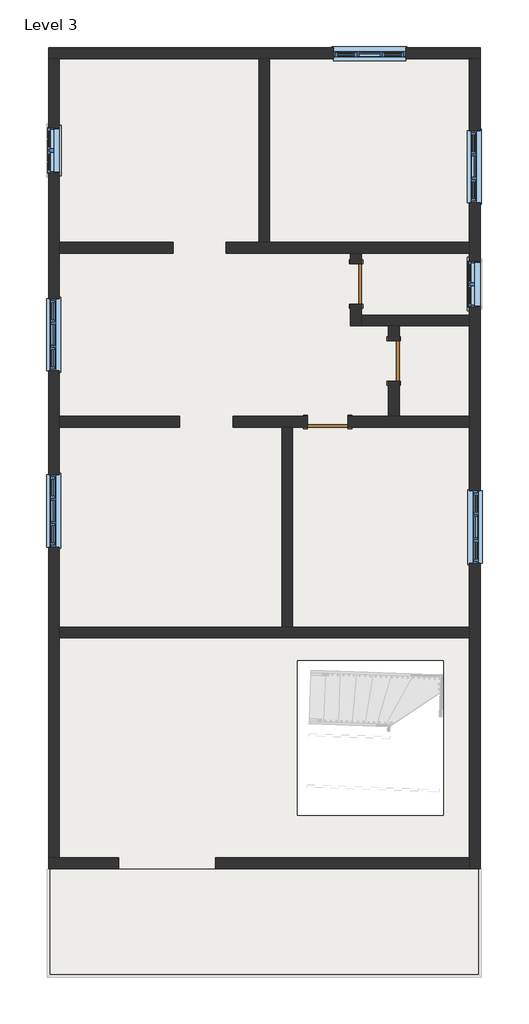
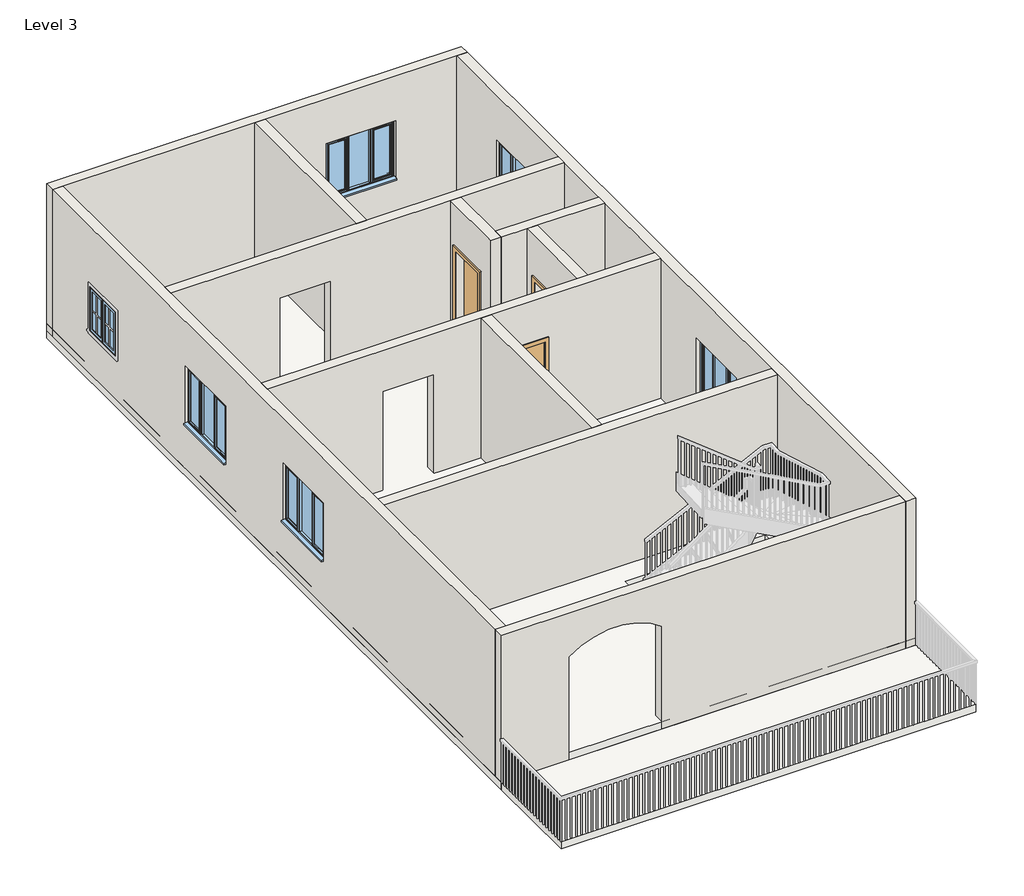
# One storey, part 1 of 3: 12 walls, 7 windows, 3 doors, 2 slabs, 1 roof.
"""IFC4 building model written with IfcOpenShell, lengths in millimetres."""

from ifc_helpers import new_model, si_unit, frame, origin, place, context, project, spatial, polyline, circle_curve, outline, extrude, faceted_brep, transform, mapped, element, save
from ifc_brep_helpers import plane_surface, revolved_surface, advanced_brep
from components import door_b6acaa4e, window_c29befe5, windows_tpl_plain_1360x1210mm_e2a6c9d8

model = new_model("IFC4")

# Units and contexts
model_context = context("Model", 3, world=origin())
ifc_project = project(units=[si_unit("LENGTHUNIT", "METRE", prefix="MILLI")], contexts=[model_context])

# Site, building, storey
site = spatial("IfcSite", under=ifc_project)
building = spatial("IfcBuilding", under=site)
storey = spatial("IfcBuildingStorey", under=building, Name="Level 3", Elevation=6096.0)

# Doors
placement = place(None, origin())
door_shape = door_b6acaa4e(model_context)
element("IfcDoor", 1, ObjectType="Single-Flush : 30\" x 84\"", at=placement, inside=storey, context=model_context, shape_type="MappedRepresentation", body=[
    mapped(door_shape, transform((-9158.3126504, 6947.728857, 6096.0), x_axis=(0.0, -1.0, 0.0), y_axis=(1.0, 0.0, 0.0), z_axis=(0.0, 0.0, 1.0))),
])
element("IfcDoor", 2, ObjectType="Single-Flush : 30\" x 84\"", at=placement, inside=storey, context=model_context, shape_type="MappedRepresentation", body=[
    mapped(door_shape, transform((-9691.7126504, 4356.928857, 6096.0), x_axis=(-1.0, 0.0, 0.0), y_axis=(0.0, -1.0, 0.0), z_axis=(0.0, 0.0, 1.0))),
])
element("IfcDoor", 3, ObjectType="Single-Flush : 30\" x 84\"", at=placement, inside=storey, context=model_context, shape_type="MappedRepresentation", body=[
    mapped(door_shape, transform((-8447.1126504, 5499.928857, 6096.0), x_axis=(0.0, -1.0, 0.0), y_axis=(1.0, 0.0, 0.0), z_axis=(0.0, 0.0, 1.0))),
])

# Roof
element("IfcRoof", 4, ObjectType="Generic - 12\"", at=placement, inside=storey, context=model_context, shape_type="SweptSolid", body=[
    extrude(outline(polyline([(-6821.5126504, -4050.471143), (-14949.5126504, -4050.471143), (-14949.5126504, 11392.728857), (-6821.5126504, 11392.728857), (-6821.5126504, -4050.471143)]), holes=[polyline([(-7518.4, -135.4836), (-10261.6, -135.4836), (-10261.6, -3048.381), (-7518.4, -3048.381), (-7518.4, -135.4836)])]), frame((0.0, 0.0, 6096.0), z_axis=(0.0, 0.0, 1.0), x_axis=(1.0, 0.0, 0.0)), (0.0, 0.0, 1.0), 152.4),
])

# Slabs
element("IfcSlab", 5, ObjectType="Generic - 12\"", at=placement, inside=storey, context=model_context, shape_type="SweptSolid", body=[
    extrude(outline(polyline([(-6821.5126504, 11392.728857), (-6821.5126504, -4050.471143), (-14949.5126504, -4050.471143), (-14949.5126504, 11392.728857), (-6821.5126504, 11392.728857)]), holes=[polyline([(-7518.4, -135.4836), (-10261.6, -135.4836), (-10261.6, -3048.381), (-7518.4, -3048.381), (-7518.4, -135.4836)])]), frame((0.0, 0.0, 5943.6), z_axis=(0.0, 0.0, 1.0), x_axis=(1.0, 0.0, 0.0)), (0.0, 0.0, 1.0), 152.4),
])
element("IfcSlab", 6, ObjectType="Generic - 12\"", at=placement, inside=storey, context=model_context, shape_type="SweptSolid", body=[
    extrude(outline(polyline([(-6821.5126504, -4050.471143), (-6821.5126504, -6082.471143), (-14949.5126504, -6082.471143), (-14949.5126504, -4050.471143), (-6821.5126504, -4050.471143)])), frame((0.0, 0.0, 5943.6), z_axis=(0.0, 0.0, 1.0), x_axis=(1.0, 0.0, 0.0)), (0.0, 0.0, 1.0), 152.4),
])

# Walls
element("IfcWall", 7, ObjectType="Generic - 4.5\" p", at=placement, inside=storey, context=model_context, shape_type="SweptSolid", body=[
    extrude(outline(polyline([(-10987.1126504, 7735.128857), (-10987.1126504, 11189.528857), (-10783.9126504, 11189.528857), (-10783.9126504, 7735.128857), (-10987.1126504, 7735.128857)])), frame((0.0, 0.0, 6096.0), z_axis=(0.0, 0.0, 1.0), x_axis=(1.0, 0.0, 0.0)), (0.0, 0.0, 1.0), 3048.0),
])
element("IfcWall", 8, ObjectType="Generic - 4.5\" p", at=placement, inside=storey, context=model_context, shape_type="Brep", body=[
    faceted_brep([(-7024.7126504, 7735.128857, 6096.0), (-10783.9126504, 7735.128857, 6096.0), (-10987.1126504, 7735.128857, 6096.0), (-11604.7126504, 7735.128857, 6096.0), (-11604.7126504, 7735.128857, 8296.0), (-12604.7126504, 7735.128857, 8296.0), (-12604.7126504, 7735.128857, 6096.0), (-14746.3126504, 7735.128857, 6096.0), (-14746.3126504, 7735.128857, 9144.0), (-10987.1126504, 7735.128857, 9144.0), (-10783.9126504, 7735.128857, 9144.0), (-7024.7126504, 7735.128857, 9144.0), (-11604.7126504, 7531.928857, 8296.0), (-11604.7126504, 7531.928857, 6096.0), (-9259.9126504, 7531.928857, 6096.0), (-9056.7126504, 7531.928857, 6096.0), (-7024.7126504, 7531.928857, 6096.0), (-7024.7126504, 7531.928857, 9144.0), (-9056.7126504, 7531.928857, 9144.0), (-9259.9126504, 7531.928857, 9144.0), (-14746.3126504, 7531.928857, 9144.0), (-14746.3126504, 7531.928857, 6096.0), (-12604.7126504, 7531.928857, 6096.0), (-12604.7126504, 7531.928857, 8296.0)], [[[0, 1, 2, 3, 4, 5, 6, 7, 8, 9, 10, 11]], [[12, 13, 14, 15, 16, 17, 18, 19, 20, 21, 22, 23]], [[22, 21, 7, 6]], [[16, 15, 14, 13, 3, 2, 1, 0]], [[11, 10, 9, 8, 20, 19, 18, 17]], [[8, 7, 21, 20]], [[0, 11, 17, 16]], [[4, 3, 13, 12]], [[5, 4, 12, 23]], [[6, 5, 23, 22]]]),
])
element("IfcWall", 9, ObjectType="Generic - 4.5\" p", at=placement, inside=storey, context=model_context, shape_type="Brep", body=[
    faceted_brep([(-9259.9126504, 6566.728857, 8229.6), (-9259.9126504, 6566.728857, 6096.0), (-9259.9126504, 6160.328857, 6096.0), (-9259.9126504, 6160.328857, 9144.0), (-9259.9126504, 7531.928857, 9144.0), (-9259.9126504, 7531.928857, 6096.0), (-9259.9126504, 7328.728857, 6096.0), (-9259.9126504, 7328.728857, 8229.6), (-9056.7126504, 6160.328857, 6096.0), (-9056.7126504, 6363.528857, 6096.0), (-9056.7126504, 6566.728857, 6096.0), (-9056.7126504, 6566.728857, 8229.6), (-9056.7126504, 7328.728857, 8229.6), (-9056.7126504, 7328.728857, 6096.0), (-9056.7126504, 7531.928857, 6096.0), (-9056.7126504, 7531.928857, 9144.0), (-9056.7126504, 6363.528857, 9144.0), (-9056.7126504, 6160.328857, 9144.0)], [[[0, 1, 2, 3, 4, 5, 6, 7]], [[8, 9, 10, 11, 12, 13, 14, 15, 16, 17]], [[6, 5, 14, 13]], [[2, 1, 10, 9, 8]], [[4, 3, 17, 16, 15]], [[5, 4, 15, 14]], [[3, 2, 8, 17]], [[11, 10, 1, 0]], [[12, 11, 0, 7]], [[13, 12, 7, 6]]]),
])
element("IfcWall", 10, ObjectType="Generic - 4.5\" p", at=placement, inside=storey, context=model_context, shape_type="Brep", body=[
    faceted_brep([(-9056.7126504, 6160.328857, 6096.0), (-8548.7126504, 6160.328857, 6096.0), (-8345.5126504, 6160.328857, 6096.0), (-7024.7126504, 6160.328857, 6096.0), (-7024.7126504, 6160.328857, 9144.0), (-8345.5126504, 6160.328857, 9144.0), (-8548.7126504, 6160.328857, 9144.0), (-9056.7126504, 6160.328857, 9144.0), (-9056.7126504, 6363.528857, 6096.0), (-9056.7126504, 6363.528857, 9144.0), (-7024.7126504, 6363.528857, 9144.0), (-7024.7126504, 6363.528857, 6096.0)], [[[0, 1, 2, 3, 4, 5, 6, 7]], [[8, 9, 10, 11]], [[3, 2, 1, 0, 8, 11]], [[7, 6, 5, 4, 10, 9]], [[0, 7, 9, 8]], [[4, 3, 11, 10]]]),
])
element("IfcWall", 11, ObjectType="Generic - 4.5\" p", at=placement, inside=storey, context=model_context, shape_type="SweptSolid", body=[
    extrude(outline(polyline([(5118.928857, 8229.6), (5118.928857, 6096.0), (4458.528857, 6096.0), (4458.528857, 9144.0), (6160.328857, 9144.0), (6160.328857, 6096.0), (5880.928857, 6096.0), (5880.928857, 8229.6), (5118.928857, 8229.6)])), frame((-8548.7126504, 0.0, 0.0), z_axis=(1.0, 0.0, 0.0), x_axis=(0.0, 1.0, 0.0)), (0.0, 0.0, 1.0), 203.2),
])
element("IfcWall", 12, ObjectType="Generic - 4.5\" p", at=placement, inside=storey, context=model_context, shape_type="Brep", body=[
    faceted_brep([(-10072.7126504, 4458.528857, 8229.6), (-10072.7126504, 4458.528857, 6096.0), (-11477.7126504, 4458.528857, 6096.0), (-11477.7126504, 4458.528857, 8296.0), (-12477.7126504, 4458.528857, 8296.0), (-12477.7126504, 4458.528857, 6096.0), (-14746.3126504, 4458.528857, 6096.0), (-14746.3126504, 4458.528857, 9144.0), (-8548.7126504, 4458.528857, 9144.0), (-8345.5126504, 4458.528857, 9144.0), (-7024.7126504, 4458.528857, 9144.0), (-7024.7126504, 4458.528857, 6096.0), (-8345.5126504, 4458.528857, 6096.0), (-8548.7126504, 4458.528857, 6096.0), (-9310.7126504, 4458.528857, 6096.0), (-9310.7126504, 4458.528857, 8229.6), (-11477.7126504, 4255.328857, 6096.0), (-10555.3126504, 4255.328857, 6096.0), (-10352.1126504, 4255.328857, 6096.0), (-10072.7126504, 4255.328857, 6096.0), (-10072.7126504, 4255.328857, 8229.6), (-9310.7126504, 4255.328857, 8229.6), (-9310.7126504, 4255.328857, 6096.0), (-7024.7126504, 4255.328857, 6096.0), (-7024.7126504, 4255.328857, 9144.0), (-10352.1126504, 4255.328857, 9144.0), (-10555.3126504, 4255.328857, 9144.0), (-14746.3126504, 4255.328857, 9144.0), (-14746.3126504, 4255.328857, 6096.0), (-12477.7126504, 4255.328857, 6096.0), (-12477.7126504, 4255.328857, 8296.0), (-11477.7126504, 4255.328857, 8296.0)], [[[0, 1, 2, 3, 4, 5, 6, 7, 8, 9, 10, 11, 12, 13, 14, 15]], [[16, 17, 18, 19, 20, 21, 22, 23, 24, 25, 26, 27, 28, 29, 30, 31]], [[29, 28, 6, 5]], [[2, 1, 19, 18, 17, 16]], [[14, 13, 12, 11, 23, 22]], [[10, 9, 8, 7, 27, 26, 25, 24]], [[11, 10, 24, 23]], [[7, 6, 28, 27]], [[3, 2, 16, 31]], [[4, 3, 31, 30]], [[5, 4, 30, 29]], [[20, 19, 1, 0]], [[21, 20, 0, 15]], [[22, 21, 15, 14]]]),
])
element("IfcWall", 13, ObjectType="Generic - 4.5\" p", at=placement, inside=storey, context=model_context, shape_type="SweptSolid", body=[
    extrude(outline(polyline([(-10555.3126504, 496.128857), (-10555.3126504, 4255.328857), (-10352.1126504, 4255.328857), (-10352.1126504, 496.128857), (-10555.3126504, 496.128857)])), frame((0.0, 0.0, 6096.0), z_axis=(0.0, 0.0, 1.0), x_axis=(1.0, 0.0, 0.0)), (0.0, 0.0, 1.0), 3048.0),
])
element("IfcWall", 14, ObjectType="Generic - 4.5\" p", at=placement, inside=storey, context=model_context, shape_type="Brep", body=[
    faceted_brep([(-14746.3126504, 292.928857, 6096.0), (-7024.7126504, 292.928857, 6096.0), (-7024.7126504, 292.928857, 9144.0), (-14746.3126504, 292.928857, 9144.0), (-14746.3126504, 496.128857, 6096.0), (-14746.3126504, 496.128857, 9144.0), (-10555.3126504, 496.128857, 9144.0), (-10352.1126504, 496.128857, 9144.0), (-7024.7126504, 496.128857, 9144.0), (-7024.7126504, 496.128857, 6096.0), (-10352.1126504, 496.128857, 6096.0), (-10555.3126504, 496.128857, 6096.0)], [[[0, 1, 2, 3]], [[4, 5, 6, 7, 8, 9, 10, 11]], [[1, 0, 4, 11, 10, 9]], [[3, 2, 8, 7, 6, 5]], [[2, 1, 9, 8]], [[0, 3, 5, 4]]]),
])
element("IfcWall", 15, ObjectType="Generic - 9\" w", at=placement, inside=storey, context=model_context, shape_type="Brep", body=[
    faceted_brep([(-14949.5126504, 11189.528857, 6096.0), (-14746.3126504, 11189.528857, 6096.0), (-10987.1126504, 11189.528857, 6096.0), (-10783.9126504, 11189.528857, 6096.0), (-7024.7126504, 11189.528857, 6096.0), (-6821.5126504, 11189.528857, 6096.0), (-6821.5126504, 11189.528857, 9144.0), (-7024.7126504, 11189.528857, 9144.0), (-10783.9126504, 11189.528857, 9144.0), (-10987.1126504, 11189.528857, 9144.0), (-14746.3126504, 11189.528857, 9144.0), (-14949.5126504, 11189.528857, 9144.0), (-8224.3126504, 11189.528857, 8220.4), (-8224.3126504, 11189.528857, 7010.4), (-9584.3126504, 11189.528857, 7010.4), (-9584.3126504, 11189.528857, 8220.4), (-14949.5126504, 11392.728857, 6096.0), (-14949.5126504, 11392.728857, 9144.0), (-6821.5126504, 11392.728857, 9144.0), (-6821.5126504, 11392.728857, 6096.0), (-8224.3126504, 11392.728857, 8220.4), (-9584.3126504, 11392.728857, 8220.4), (-9584.3126504, 11392.728857, 7010.4), (-8224.3126504, 11392.728857, 7010.4)], [[[0, 1, 2, 3, 4, 5, 6, 7, 8, 9, 10, 11], [12, 13, 14, 15]], [[16, 17, 18, 19], [20, 21, 22, 23]], [[5, 4, 3, 2, 1, 0, 16, 19]], [[11, 10, 9, 8, 7, 6, 18, 17]], [[6, 5, 19, 18]], [[0, 11, 17, 16]], [[13, 12, 20, 23]], [[14, 13, 23, 22]], [[15, 14, 22, 21]], [[12, 15, 21, 20]]]),
])
element("IfcWall", 16, ObjectType="Generic - 9\" w", at=placement, inside=storey, context=model_context, shape_type="Brep", body=[
    faceted_brep([(-7024.7126504, 11189.528857, 6096.0), (-7024.7126504, 7735.128857, 6096.0), (-7024.7126504, 7531.928857, 6096.0), (-7024.7126504, 6363.528857, 6096.0), (-7024.7126504, 6160.328857, 6096.0), (-7024.7126504, 4458.528857, 6096.0), (-7024.7126504, 4255.328857, 6096.0), (-7024.7126504, 496.128857, 6096.0), (-7024.7126504, 292.928857, 6096.0), (-7024.7126504, -3847.271143, 6096.0), (-7024.7126504, -4050.471143, 6096.0), (-7024.7126504, -4050.471143, 9144.0), (-7024.7126504, -3847.271143, 9144.0), (-7024.7126504, 292.928857, 9144.0), (-7024.7126504, 496.128857, 9144.0), (-7024.7126504, 4255.328857, 9144.0), (-7024.7126504, 4458.528857, 9144.0), (-7024.7126504, 6160.328857, 9144.0), (-7024.7126504, 6363.528857, 9144.0), (-7024.7126504, 7531.928857, 9144.0), (-7024.7126504, 7735.128857, 9144.0), (-7024.7126504, 11189.528857, 9144.0), (-7024.7126504, 8477.528857, 8220.4), (-7024.7126504, 8477.528857, 7010.4), (-7024.7126504, 9837.528857, 7010.4), (-7024.7126504, 9837.528857, 8220.4), (-7024.7126504, 3055.728857, 8220.4), (-7024.7126504, 1695.728857, 8220.4), (-7024.7126504, 1695.728857, 7010.4), (-7024.7126504, 3055.728857, 7010.4), (-7024.7126504, 7379.528857, 7924.8), (-7024.7126504, 6515.928857, 7924.8), (-7024.7126504, 6515.928857, 7010.4), (-7024.7126504, 7379.528857, 7010.4), (-6821.5126504, 11189.528857, 6096.0), (-6821.5126504, 11189.528857, 9144.0), (-6821.5126504, -4050.471143, 9144.0), (-6821.5126504, -4050.471143, 6096.0), (-6821.5126504, 8477.528857, 8220.4), (-6821.5126504, 9837.528857, 8220.4), (-6821.5126504, 9837.528857, 7010.4), (-6821.5126504, 8477.528857, 7010.4), (-6821.5126504, 3055.728857, 8220.4), (-6821.5126504, 3055.728857, 7010.4), (-6821.5126504, 1695.728857, 7010.4), (-6821.5126504, 1695.728857, 8220.4), (-6821.5126504, 7379.528857, 7924.8), (-6821.5126504, 7379.528857, 7010.4), (-6821.5126504, 6515.928857, 7010.4), (-6821.5126504, 6515.928857, 7924.8)], [[[0, 1, 2, 3, 4, 5, 6, 7, 8, 9, 10, 11, 12, 13, 14, 15, 16, 17, 18, 19, 20, 21], [22, 23, 24, 25], [26, 27, 28, 29], [30, 31, 32, 33]], [[34, 35, 36, 37], [38, 39, 40, 41], [42, 43, 44, 45], [46, 47, 48, 49]], [[10, 9, 8, 7, 6, 5, 4, 3, 2, 1, 0, 34, 37]], [[21, 20, 19, 18, 17, 16, 15, 14, 13, 12, 11, 36, 35]], [[0, 21, 35, 34]], [[11, 10, 37, 36]], [[23, 22, 38, 41]], [[24, 23, 41, 40]], [[25, 24, 40, 39]], [[22, 25, 39, 38]], [[43, 42, 26, 29]], [[44, 43, 29, 28]], [[45, 44, 28, 27]], [[42, 45, 27, 26]], [[47, 46, 30, 33]], [[48, 47, 33, 32]], [[49, 48, 32, 31]], [[46, 49, 31, 30]]]),
])
element("IfcWall", 17, ObjectType="Generic - 9\" w", at=placement, inside=storey, context=model_context, shape_type="AdvancedBrep", body=[
    advanced_brep(
    [(-14949.5126504, -3847.271143, 9144.0), (-14746.3126504, -3847.271143, 9144.0), (-7024.7126504, -3847.271143, 9144.0), (-7024.7126504, -3847.271143, 6096.0), (-11799.9126504, -3847.271143, 6096.0), (-11799.9126504, -3847.271143, 8229.6), (-13628.7126504, -3847.271143, 8229.6), (-13628.7126504, -3847.271143, 6096.0), (-14746.3126504, -3847.271143, 6096.0), (-14949.5126504, -3847.271143, 6096.0), (-7024.7126504, -4050.471143, 9144.0), (-14949.5126504, -4050.471143, 9144.0), (-14949.5126504, -4050.471143, 6096.0), (-13628.7126504, -4050.471143, 6096.0), (-13628.7126504, -4050.471143, 8229.6), (-11799.9126504, -4050.471143, 8229.6), (-11799.9126504, -4050.471143, 6096.0), (-7024.7126504, -4050.471143, 6096.0)],
    [
        (0, 1),
        (1, 2),
        (2, 3),
        (3, 4),
        (4, 5),
        (5, 6, circle_curve(frame((-12714.3126504, -3847.271143, 7013.0443508), z_axis=(0.0, -1.0, 0.0), x_axis=(1.0, 0.0, 0.0)), 1521.8853464)),
        (6, 7),
        (7, 8),
        (8, 9),
        (9, 0),
        (10, 11),
        (11, 12),
        (12, 13),
        (13, 14),
        (14, 15, circle_curve(frame((-12714.3126504, -4050.471143, 7013.0443508), z_axis=(0.0, 1.0, 0.0), x_axis=(1.0, 0.0, 0.0)), 1521.8853464)),
        (15, 16),
        (16, 17),
        (17, 10),
        (3, 17),
        (16, 4),
        (12, 9),
        (7, 13),
        (0, 11),
        (10, 2),
        (15, 5),
        (14, 6),
    ],
    [
        plane_surface(frame((-6923.1126504, -3847.271143, 6096.0), z_axis=(0.0, 1.0, 0.0), x_axis=(-1.0, 0.0, 0.0))),
        plane_surface(frame((-6923.1126504, -4050.471143, 6096.0), z_axis=(0.0, -1.0, 0.0), x_axis=(1.0, 0.0, 0.0))),
        plane_surface(frame((-6923.1126504, -3847.271143, 6096.0), z_axis=(0.0, 0.0, -1.0), x_axis=(0.0, -1.0, 0.0))),
        plane_surface(frame((-14847.9126504, -3847.271143, 9144.0), z_axis=(0.0, 0.0, 1.0), x_axis=(0.0, -1.0, 0.0))),
        plane_surface(frame((-7024.7126504, 11291.128857, 6096.0), z_axis=(1.0, 0.0, 0.0), x_axis=(0.0, -1.0, 0.0))),
        plane_surface(frame((-14949.5126504, -3948.871143, 6096.0), z_axis=(-1.0, 0.0, 0.0), x_axis=(0.0, -1.0, 0.0))),
        plane_surface(frame((-11799.9126504, -5574.471143, 6096.0), z_axis=(-1.0, 0.0, 0.0), x_axis=(0.0, 1.0, 0.0))),
        revolved_surface(polyline([(-11192.427303999999, -4050.471143, 7013.0443508), (-11192.427303999999, -3847.271143, 7013.0443508)]), (-12714.3126504, -2526.471143, 7013.0443508), (0.0, -1.0, 0.0)),
        plane_surface(frame((-13628.7126504, -5574.471143, 8229.6), z_axis=(1.0, 0.0, 0.0), x_axis=(0.0, 1.0, 0.0))),
    ],
    [
        (0, [[1, 2, 3, 4, 5, 6, 7, 8, 9, 10]]),
        (1, [[11, 12, 13, 14, 15, 16, 17, 18]]),
        (2, [[19, -17, 20, -4]]),
        (2, [[21, -9, -8, 22, -13]]),
        (3, [[-2, -1, 23, -11, 24]]),
        (4, [[-3, -24, -18, -19]]),
        (5, [[-10, -21, -12, -23]]),
        (6, [[25, -5, -20, -16]]),
        (7, [[-25, -15, 26, -6]]),
        (8, [[-26, -14, -22, -7]]),
    ],
),
])
element("IfcWall", 18, ObjectType="Generic - 9\" w", at=placement, inside=storey, context=model_context, shape_type="Brep", body=[
    faceted_brep([(-14746.3126504, -3847.271143, 6096.0), (-14746.3126504, 292.928857, 6096.0), (-14746.3126504, 496.128857, 6096.0), (-14746.3126504, 4255.328857, 6096.0), (-14746.3126504, 4458.528857, 6096.0), (-14746.3126504, 7531.928857, 6096.0), (-14746.3126504, 7735.128857, 6096.0), (-14746.3126504, 11189.528857, 6096.0), (-14746.3126504, 11189.528857, 9144.0), (-14746.3126504, 7735.128857, 9144.0), (-14746.3126504, 7531.928857, 9144.0), (-14746.3126504, 4458.528857, 9144.0), (-14746.3126504, 4255.328857, 9144.0), (-14746.3126504, 496.128857, 9144.0), (-14746.3126504, 292.928857, 9144.0), (-14746.3126504, -3847.271143, 9144.0), (-14746.3126504, 5315.228857, 8220.4), (-14746.3126504, 6675.228857, 8220.4), (-14746.3126504, 6675.228857, 7010.4), (-14746.3126504, 5315.228857, 7010.4), (-14746.3126504, 2000.528857, 8220.4), (-14746.3126504, 3360.528857, 8220.4), (-14746.3126504, 3360.528857, 7010.4), (-14746.3126504, 2000.528857, 7010.4), (-14746.3126504, 9894.128857, 7924.8), (-14746.3126504, 9894.128857, 7010.4), (-14746.3126504, 9030.528857, 7010.4), (-14746.3126504, 9030.528857, 7924.8), (-14949.5126504, -3847.271143, 6096.0), (-14949.5126504, -3847.271143, 9144.0), (-14949.5126504, 11189.528857, 9144.0), (-14949.5126504, 11189.528857, 6096.0), (-14949.5126504, 5315.228857, 8220.4), (-14949.5126504, 5315.228857, 7010.4), (-14949.5126504, 6675.228857, 7010.4), (-14949.5126504, 6675.228857, 8220.4), (-14949.5126504, 2000.528857, 8220.4), (-14949.5126504, 2000.528857, 7010.4), (-14949.5126504, 3360.528857, 7010.4), (-14949.5126504, 3360.528857, 8220.4), (-14949.5126504, 9894.128857, 7924.8), (-14949.5126504, 9030.528857, 7924.8), (-14949.5126504, 9030.528857, 7010.4), (-14949.5126504, 9894.128857, 7010.4)], [[[0, 1, 2, 3, 4, 5, 6, 7, 8, 9, 10, 11, 12, 13, 14, 15], [16, 17, 18, 19], [20, 21, 22, 23], [24, 25, 26, 27]], [[28, 29, 30, 31], [32, 33, 34, 35], [36, 37, 38, 39], [40, 41, 42, 43]], [[7, 6, 5, 4, 3, 2, 1, 0, 28, 31]], [[15, 14, 13, 12, 11, 10, 9, 8, 30, 29]], [[8, 7, 31, 30]], [[0, 15, 29, 28]], [[33, 32, 16, 19]], [[34, 33, 19, 18]], [[35, 34, 18, 17]], [[32, 35, 17, 16]], [[37, 36, 20, 23]], [[38, 37, 23, 22]], [[39, 38, 22, 21]], [[36, 39, 21, 20]], [[25, 24, 40, 43]], [[26, 25, 43, 42]], [[27, 26, 42, 41]], [[24, 27, 41, 40]]]),
])

# Windows
window_shape = window_c29befe5(model_context)
element("IfcWindow", 19, ObjectType="Window-Casement-Double : 34\" x 36\"", at=placement, inside=storey, context=model_context, shape_type="MappedRepresentation", body=[
    mapped(window_shape, transform((-14847.9126504, 9462.328857, 6096.0), x_axis=(0.0, 1.0, 0.0), y_axis=(-1.0, 0.0, 0.0), z_axis=(0.0, 0.0, 1.0))),
])
element("IfcWindow", 20, ObjectType="Window-Casement-Double : 34\" x 36\"", at=placement, inside=storey, context=model_context, shape_type="MappedRepresentation", body=[
    mapped(window_shape, transform((-6923.1126504, 6947.728857, 6096.0), x_axis=(0.0, 1.0, 0.0), y_axis=(-1.0, 0.0, 0.0), z_axis=(0.0, 0.0, 1.0))),
])
windows_tpl_plain_1360x1210mm_shape = windows_tpl_plain_1360x1210mm_e2a6c9d8(model_context)
element("IfcWindow", 21, ObjectType="Windows_Tpl_Plain : 1360x1210mm", at=placement, inside=storey, context=model_context, shape_type="MappedRepresentation", body=[
    mapped(windows_tpl_plain_1360x1210mm_shape, transform((-9405.979317, 11299.5854248, 6110.4), x_axis=(-1.0, 0.0, 0.0), y_axis=(0.0, -1.0, 0.0), z_axis=(0.0, 0.0, 1.0))),
])
element("IfcWindow", 22, ObjectType="Windows_Tpl_Plain : 1360x1210mm", at=placement, inside=storey, context=model_context, shape_type="MappedRepresentation", body=[
    mapped(windows_tpl_plain_1360x1210mm_shape, transform((-6914.6560825, 9659.1955236, 6110.4), x_axis=(0.0, 1.0, 0.0), y_axis=(-1.0, 0.0, 0.0), z_axis=(0.0, 0.0, 1.0))),
])
element("IfcWindow", 23, ObjectType="Windows_Tpl_Plain : 1360x1210mm", at=placement, inside=storey, context=model_context, shape_type="MappedRepresentation", body=[
    mapped(windows_tpl_plain_1360x1210mm_shape, transform((-6931.5692182, 1874.0621903, 6110.4), x_axis=(0.0, -1.0, 0.0), y_axis=(1.0, 0.0, 0.0), z_axis=(0.0, 0.0, 1.0))),
])
element("IfcWindow", 24, ObjectType="Windows_Tpl_Plain : 1360x1210mm", at=placement, inside=storey, context=model_context, shape_type="MappedRepresentation", body=[
    mapped(windows_tpl_plain_1360x1210mm_shape, transform((-14839.4560825, 6496.8955236, 6110.4), x_axis=(0.0, 1.0, 0.0), y_axis=(-1.0, 0.0, 0.0), z_axis=(0.0, 0.0, 1.0))),
])
element("IfcWindow", 25, ObjectType="Windows_Tpl_Plain : 1360x1210mm", at=placement, inside=storey, context=model_context, shape_type="MappedRepresentation", body=[
    mapped(windows_tpl_plain_1360x1210mm_shape, transform((-14839.4560825, 3182.1955236, 6110.4), x_axis=(0.0, 1.0, 0.0), y_axis=(-1.0, 0.0, 0.0), z_axis=(0.0, 0.0, 1.0))),
])

save(model, "model.ifc")

# Revit data of these elements
# Type "Single-Flush : 30\" x 84\""
#   Type Mark = "4"
#   Construction Type Id = "MDOOR"
#   Assembly Code = "C1020"
#   Analytic Construction = "Metal"
#   Thickness = 0' - 2"
#   Heat Transfer Coefficient (U) = 0.651978 BTU/(h·ft²·°F)
#   Height = 7' - 0"
#   Trim Projection Ext = 0' - 1"
#   Trim Projection Int = 0' - 1"
#   Trim Width = 0' - 3"
#   Width = 2' - 6"
#   Define Thermal Properties by = 1
#   Define Thermal Properties by = 1
#   Door Material = Door - Panel
#   Frame Material = Door - Frame
#   Visual Light Transmittance = 0
#   Solar Heat Gain Coefficient = 0
#   Function = (empty or 0)
#   Wall Closure = (empty or 0)
# Type "Generic - 12\""
#   Assembly Code = "B1020"
#   Layers, outside or top first: 0' - 6" no material (function 1)
# Type "Generic - 12\""
#   Assembly Code = "B1010"
#   Function = 0
#   Layers, outside or top first: 0' - 6" no material (function 1)
# Type "Generic - 4.5\" p"
#   Assembly Code = "B2010"
#   Layers, outside or top first: 0' - 8" "Brick, Common" (function 1)
# Type "Generic - 9\" w"
#   Assembly Code = "B2010"
#   Layers, outside or top first: 0' - 8" no material (function 1)
# Type "Window-Casement-Double : 34\" x 36\""
#   Type Mark = "14"
#   Fire Rating = "0.5h"
#   Assembly Code = "B2020100"
#   Analytic Construction = "Double glazing - domestic"
#   Frame Extension [instance default] = 0' - 0 1/4"
#   Window Inset [instance default] = 0' - 0"
#   Wall Thickness [instance default] = 0' - 6"
#   Interior Wall Closure [instance default] = 0' - 2 1/4"
#   Half Width = 1' - 5"
#   Visual Light Transmittance = 0.81
#   Thermal Resistance (R) = 1.8146 (h·ft²·°F)/BTU
#   Solar Heat Gain Coefficient = 0.76
#   Rough Width = 2' - 10 1/2"
#   Rough Height = 3' - 0 1/2"
#   Height = 3' - 0"
#   Heat Transfer Coefficient (U) = 0.5511 BTU/(h·ft²·°F)
#   Exterior Wall Closure [instance default] = 0' - 1 1/4"
#   Extension Jamb [instance default] = 0' - 2 1/4"
#   Default Sill Height = 3' - 0"
#   Width = 2' - 10"
#   Define Thermal Properties by = 0
#   Muntin Visibility = yes
#   Interior Trim Visibility [instance default] = yes
#   Exterior Trim Visibility [instance default] = yes
#   Extension Jamb Visibility [instance default] = yes
#   Interior Trim Material = Wood - Stained
#   Muntin Pattern = Muntin Pattern_2x2 : Muntin Pattern_2x2
#   Interior Trim = Trim-Window-Interior-Flat : Picture Frame
#   Interior Frame Material = Wood - Stained
#   Glass Panel Material = Glass
#   Exterior Trim Material = Clad - White
#   Exterior Trim = Trim-Window-Exterior-Flat : with Sill
#   Exterior Frame Material = Clad - White
#   Wall Closure = (empty or 0)
# Type "Windows_Tpl_Plain : 1360x1210mm"
#   Type Mark = "21"
#   Operation = "TriplePanelVertical"
#   Construction Type Id = "GSP4R"
#   Manufacturer = "Revit"
#   Keynote = "L10"
#   Analytic Construction = "1/8 in Pilkington single glazing"
#   Wrap Layers (Ext) from Ext = 0' - 4.03543"
#   Wrap Layers (Int) from Ext = 0' - 6.98819"
#   Window Board Projection = 0' - 0.98425"
#   Window Board Extension = 0' - 0.98425"
#   Visual Light Transmittance = 0.9
#   Solar Heat Gain Coefficient = 0.78
#   Rough Width = 4' - 5.54331"
#   Rough Height = 3' - 11.6378"
#   Height = 3' - 11.6378"
#   Width = 4' - 5.54331"
#   Heat Transfer Coefficient (U) = 0.6496 BTU/(h·ft²·°F)
#   Glazing Thickness = 0' - 0.94488"
#   FrameOffset - External = 0' - 1.9685"
#   Frame Depth = 0' - 2.55906"
#   Default Head Height = 6' - 11.07087"
#   Cill Depth = 0' - 3.44488"
#   Cavity Closer Width = 0' - 1.9685"
#   Cavity Closer Offset from Ext = 0' - 4.03543"
#   Cavity Closer Depth = 0' - 3.34646"
#   Vis - Cavity Closers = yes
#   Define Thermal Properties by = 1
#   Material Trim = Window Frame
#   Material Glass = Glass
#   Material Frame = Window Frame
#   Wall Closure = (empty or 0)
# Elements 1, 2, 3 (IfcDoor, "Single-Flush : 30\" x 84\"")
#   Phase Created = New Construction
#   Materials on its faces: "Door - Frame", "Door - Panel"
# Element 4 (IfcRoof, "Generic - 12\"")
#   built-in parameter 1001705 = 20.5 (stored number, unit not read)
#   built-in parameter 1001710 = 33615
#   Phase Created = New Construction
#   Materials on its faces: "Default Roof"
# Element 5 (IfcSlab, "Generic - 12\"")
#   Height Offset From Level = 0' - 0"
#   Phase Created = New Construction
#   Materials on its faces: "Default Floor"
# Element 6 (IfcSlab, "Generic - 12\"")
#   Height Offset From Level = 0' - 0"
#   Phase Created = New Construction
#   Materials on its faces: "Default Floor", "Brick, Soldier Course"
# Elements 7, 8, 9, 11, 12, 13 (IfcWall, "Generic - 4.5\" p")
#   Top Offset = 0' - 0"
#   Base Offset = 0' - 0"
#   wall height = 10' - 0"
#   Phase Created = New Construction
#   Base Constraint = Level 3
#   Top Constraint = Level 4
#   Materials on its faces: "Brick, Common", "Cherry"
# Elements 10, 14 (IfcWall, "Generic - 4.5\" p")
#   Top Offset = 0' - 0"
#   Base Offset = 0' - 0"
#   wall height = 10' - 0"
#   Phase Created = New Construction
#   Base Constraint = Level 3
#   Top Constraint = Level 4
#   Materials on its faces: "Brick, Common"
# Elements 15, 18 (IfcWall, "Generic - 9\" w")
#   Top Offset = 0' - 0"
#   Base Offset = 0' - 0"
#   wall height = 10' - 0"
#   Phase Created = New Construction
#   Base Constraint = Level 3
#   Top Constraint = Level 4
#   Materials on its faces: "Default Wall", "Cherry"
# Element 16 (IfcWall, "Generic - 9\" w")
#   Top Offset = 0' - 0"
#   Base Offset = 0' - 0"
#   wall height = 10' - 0"
#   Phase Created = New Construction
#   Base Constraint = Level 3
#   Top Constraint = Level 4
#   Materials on its faces: "Default Wall", "Cherry", "Brick, Common"
# Element 17 (IfcWall, "Generic - 9\" w")
#   Top Offset = 0' - 0"
#   Base Offset = 0' - 0"
#   wall height = 10' - 0"
#   Phase Created = New Construction
#   Base Constraint = Level 3
#   Top Constraint = Level 4
#   Materials on its faces: "Default Wall", "Brick, Common"
# Element 19 (IfcWindow, "Window-Casement-Double : 34\" x 36\"")
#   Mark = "34"
#   Window Inset = 0' - 0"
#   Interior Wall Closure = 0' - 2 1/4"
#   Frame Extension = 0' - 0 1/4"
#   Exterior Wall Closure = 0' - 1 1/4"
#   Interior Trim Visibility = yes
#   Exterior Trim Visibility = yes
#   Phase Created = New Construction
#   Materials on its faces: "Wood - Stained", "Glass", "Clad - White"
# Element 20 (IfcWindow, "Window-Casement-Double : 34\" x 36\"")
#   Mark = "35"
#   Window Inset = 0' - 0"
#   Interior Wall Closure = 0' - 2 1/4"
#   Frame Extension = 0' - 0 1/4"
#   Exterior Wall Closure = 0' - 1 1/4"
#   Interior Trim Visibility = yes
#   Exterior Trim Visibility = yes
#   Phase Created = New Construction
#   Materials on its faces: "Wood - Stained", "Glass", "Clad - White"
# Element 21 (IfcWindow, "Windows_Tpl_Plain : 1360x1210mm")
#   Mark = "29"
#   Phase Created = New Construction
#   Materials on its faces: "Window Frame", "Glass"
# Element 22 (IfcWindow, "Windows_Tpl_Plain : 1360x1210mm")
#   Mark = "30"
#   Phase Created = New Construction
#   Materials on its faces: "Window Frame", "Glass"
# Element 23 (IfcWindow, "Windows_Tpl_Plain : 1360x1210mm")
#   Mark = "31"
#   Phase Created = New Construction
#   Materials on its faces: "Window Frame", "Glass"
# Element 24 (IfcWindow, "Windows_Tpl_Plain : 1360x1210mm")
#   Mark = "32"
#   Phase Created = New Construction
#   Materials on its faces: "Window Frame", "Glass"
# Element 25 (IfcWindow, "Windows_Tpl_Plain : 1360x1210mm")
#   Mark = "33"
#   Phase Created = New Construction
#   Materials on its faces: "Window Frame", "Glass"
# Materials
#   "Door - Panel": class "Wood", colour RGB 210 159 95, transparency 0, Cost = 0
#   "Door - Frame": colour RGB 118 70 51, transparency 0, Cost = 0
#   "Brick, Common": class "Masonry", colour RGB 128 0 128, transparency 0, Description = "Common brick", Cost = 0
#   "Wood - Stained": class "Wood", colour RGB 224 178 126, transparency 0, Cost = 0
#   "Glass": class "Glass", colour RGB 0 128 192, transparency 0.75, Description = "Soda Lime Glass", Cost = 0
#   "Clad - White": class "Wood", colour RGB 242 242 238, transparency 0, Cost = 0
#   "Window Frame": colour RGB 249 249 249, transparency 0
#   "Default Roof": colour RGB 88 101 114, transparency 0, Cost = 0
#   "Default Floor": colour RGB 128 128 128, transparency 0, Cost = 0
#   "Brick, Soldier Course": class "Masonry", colour RGB 170 98 104, transparency 0, Description = "Common brick soldier coursed", Cost = 0
#   "Cherry": class "Wood", colour RGB 226 177 128, transparency 0, Description = "Prunus Serotina", Cost = 0
#   "Default Wall": colour RGB 128 128 128, transparency 0, Cost = 0
